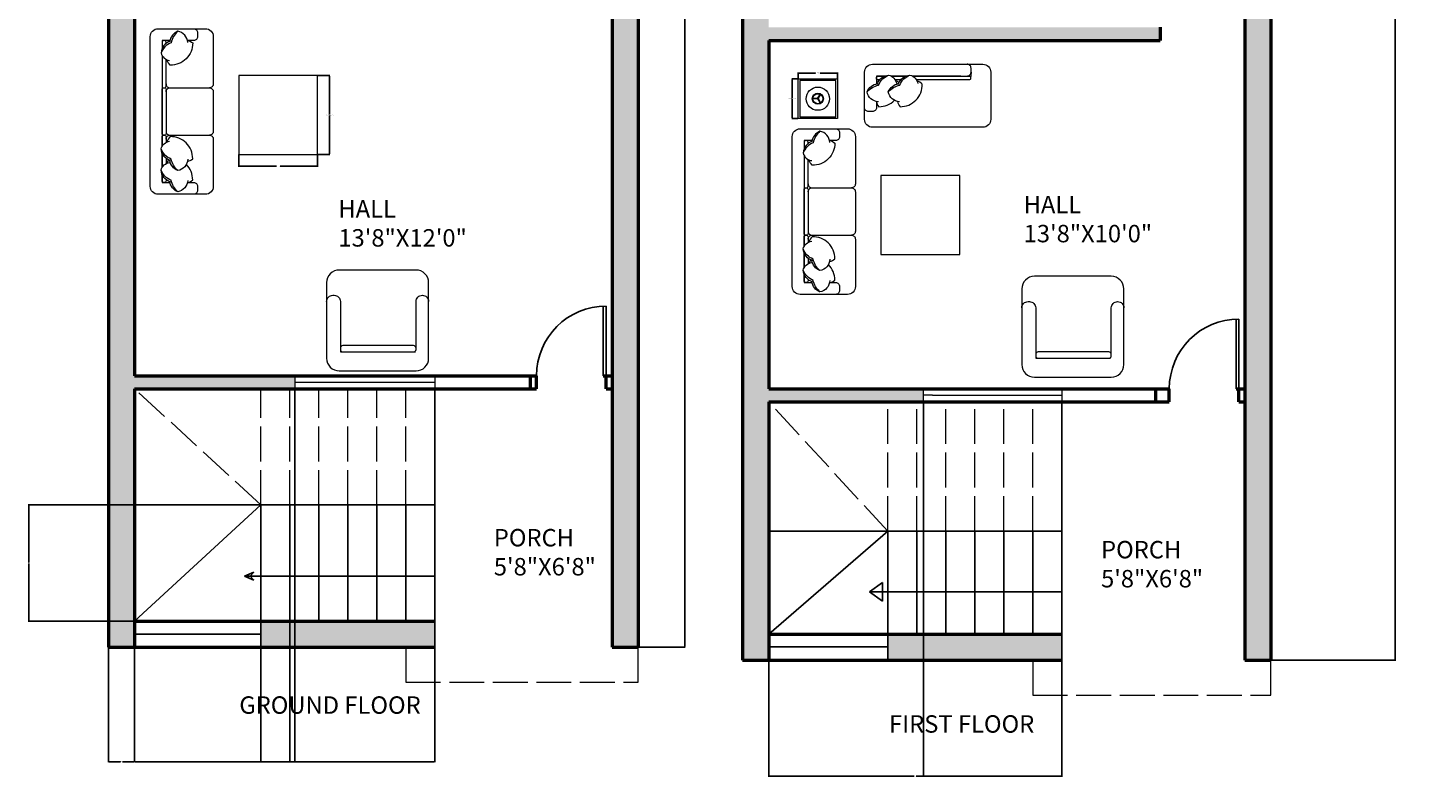
# Model space of a CAD drawing. Units: inches. Extents: x 3 to 485, y -522 to 42.
# Tile 1 of 6: x 3 to 485, y -522 to -264. Entities that reach past the tile are written whole.
import ezdxf

# ---------------------------------------------------------------- set-up
doc = ezdxf.new("R2010")
doc.units = ezdxf.units.IN
doc.header["$MEASUREMENT"] = 0
doc.linetypes.add('ACAD_ISO02W100', pattern=[15, 12, -3])
for name, color, linetype, lineweight in [('A-ANNO-DIMS', 2, 'Continuous', 18), ('A-ANNO-TEXT', 7, 'Continuous', 25), ('A-AREA-IDEN', 7, 'Continuous', 18), ('A-DOOR', 3, 'Continuous', 25), ('A-FLOR-OVHD', 7, 'ACAD_ISO02W100', 18), ('A-FLOR-STRS', 7, 'Continuous', 25), ('A-FLOR-STRS-OVHD', 7, 'ACAD_ISO02W100', 18), ('A-FURN', 8, 'Continuous', 18), ('A-GLAZ', 4, 'Continuous', 18), ('A-WALL', 7, 'Continuous', 50)]:
    doc.layers.add(name, color=color, linetype=linetype, lineweight=lineweight)
doc.layers.add('A-WALL-PATT', color=18, linetype='Continuous', lineweight=13, true_color=0x000000)
doc.styles.get("Standard").update_dxf_attribs({"font": 'arial.ttf'})
doc.dimstyles.get("Standard").update_dxf_attribs({"dimtxt": 0.18, "dimasz": 0.18, "dimexe": 0.18, "dimexo": 0.0625, "dimgap": 0.09, "dimtad": 0, "dimtih": 1, "dimtoh": 1, "dimdec": 0, "dimzin": 0, "dimdsep": 46, "dimlunit": 3, "dimtxsty": 'Standard', "dimcen": 0.09, "dimadec": 0, "dimazin": 0, "dimtfac": 1, "dimtdec": 0, "dimtofl": 0, "dimtmove": 0, "dimatfit": 3, "dimfxl": 1, "dimtolj": 1, "dimtzin": 0, "dimarcsym": 0})

# ---------------------------------------------------------------- blocks, each defined once
blk = doc.blocks.new('*D5')
at = {"layer": 'A-ANNO-DIMS', "color": 0, "lineweight": -2, "transparency": 16777216}
for p, q in [((212.85, 14), (229.02, 14)), ((228.84, 13.82), (228.84, -228.64)), ((228.84, -477.32), (228.84, -234.85)), ((212.85, -477.5), (229.02, -477.5))]:
    blk.add_line(p, q, dxfattribs=at)
at = {"layer": 'A-ANNO-DIMS', "color": 0, "transparency": 16777216}
for points in [[(228.81, 13.82), (228.87, 13.82), (228.84, 14)], [(228.81, -477.32), (228.87, -477.32), (228.84, -477.5)]]:
    blk.add_solid(points, dxfattribs=at)
at = {"layer": 'Defpoints', "color": 0, "transparency": 16777216}
for p in [(212.79, 14), (212.79, -477.5), (228.84, -477.5)]:
    blk.add_point(p, dxfattribs=at)
at = {"layer": 'A-ANNO-DIMS', "color": 0, "transparency": 16777216, "insert": (228.84, -231.75), "char_height": 6, "attachment_point": 5}
blk.add_mtext("\\A1;41'", dxfattribs=at)
blk = doc.blocks.new('DAY BED1')
at = {"color": 0}
blk.add_line((0.3, 0.25), (0.225, 0.255), dxfattribs=at)
blk.add_lwpolyline([(-0.3, 0, -0.414214), (-0.4, 0.1), (-0.4, 0.1, 0.317837), (-0.4, 0.1, -0.414214), (-0.4, 0.1), (-0.4, 0.1, 1.186185), (-0.4, 0.1, -0.414214), (-0.4, 0.1), (-0.4, 1.5, -0.414214), (-0.3, 1.6), (0.3, 1.6, -0.414214), (0.4, 1.5), (0.4, 0.1, -0.414214), (0.3, 0)], format="xyb", close=True, dxfattribs=at)
for points in [[(-0.073, 1.45), (-0.15, 1.45, -0.414214), (-0.2, 1.5), (-0.2, 1.55, -0.414214), (-0.15, 1.6)], [(-0.073, 1.45, 0.165541), (-0.139, 1.419, 0.200231), (-0.058, 1.221, 0.121523)], [(-0.076, 1.425, -0.356772), (0.05, 1.568, -0.249542), (0.154, 1.438, 9.61688)], [(0.05, 1.568, -0.14773), (0.136, 1.422, -0.213343), (0.262, 1.293, -0.178662)], [(0.143, 1.442, -0.306663), (0.262, 1.293, -0.30633), (0.154, 1.196, 0.872847)], [(0.25, 1.345), (0.25, 1.45), (0.152, 1.45, -0.414214)], [(0.2, 1.412), (0.2, 1.43, -0.414214), (0.22, 1.45), (0.23, 1.45, -0.414214), (0.25, 1.43)], [(0.25, 1.43), (0.25, 1.345, -0.414214)], [(-0.076, 1.156, -0.356772), (0.05, 1.299, -0.249542), (0.154, 1.169, 9.61688)], [(0.05, 1.299, -0.14773), (0.136, 1.153, -0.213343), (0.262, 1.024, -0.178662)], [(0.25, 1.262), (0.25, 1.075, -0.414214)], [(-0.073, 1.181, 0.165541), (-0.139, 1.15, 0.425989), (0.148, 0.869, 0.121523), (0.187, 0.936, -7.115464)], [(0.143, 1.173, -0.306663), (0.262, 1.024, -0.30633), (0.154, 0.926, 0.872847)], [(0.168, 1.163, 0.071865), (0.187, 1.205, -7.115464)], [(0.2, 1.142), (0.2, 1.211, -0.414214)], [(0.25, 0.992), (0.25, 0.275, -0.414214), (0.23, 0.255), (0.22, 0.255, -0.414214), (0.2, 0.275), (0.2, 0.942, -0.414214)], [(0.25, 0.377), (0.25, 0.3, 0.414214), (0.3, 0.25), (0.35, 0.25, 0.414214), (0.4, 0.3)]]:
    blk.add_lwpolyline(points, format="xyb", dxfattribs=at)
for points in [[(0.25, 1.075), (0.25, 1.262)], [(0.25, 0.377), (0.25, 0.992)]]:
    blk.add_lwpolyline(points, dxfattribs=at)
blk = doc.blocks.new('*D7')
at = {"layer": 'A-ANNO-DIMS', "color": 0, "lineweight": -2, "transparency": 16777216}
for p, q in [((430.85, 14), (473.81, 14)), ((473.63, 13.82), (473.63, -230.89)), ((473.63, -481.82), (473.63, -237.1)), ((430.85, -482), (473.81, -482))]:
    blk.add_line(p, q, dxfattribs=at)
at = {"layer": 'A-ANNO-DIMS', "color": 0, "transparency": 16777216}
for points in [[(473.6, 13.82), (473.66, 13.82), (473.63, 14)], [(473.6, -481.82), (473.66, -481.82), (473.63, -482)]]:
    blk.add_solid(points, dxfattribs=at)
at = {"layer": 'Defpoints', "color": 0, "transparency": 16777216}
for p in [(430.79, 14), (430.79, -482), (473.63, -482)]:
    blk.add_point(p, dxfattribs=at)
at = {"layer": 'A-ANNO-DIMS', "color": 0, "transparency": 16777216, "insert": (473.63, -234), "char_height": 6, "attachment_point": 5}
blk.add_mtext('\\A1;41\'-4"', dxfattribs=at)
blk = doc.blocks.new('LIVING-SIDE-TABLE')
for p, q in [((6.79, 6.87), (4.87, 6.87)), ((6.79, 6.7), (4.87, 6.7)), ((6.72, 6.83), (7.67, 8.49)), ((6.72, 6.75), (7.67, 5.09)), ((6.86, 6.75), (7.82, 8.41)), ((6.86, 6.83), (7.82, 5.17))]:
    blk.add_line(p, q)
at = {"ltscale": 0.03}
blk.add_lwpolyline([(13.58, 13.58), (13.58, 0), (0, 0), (0, 13.58)], close=True, dxfattribs=at)
blk.add_lwpolyline([(13.04, 0.54), (13.04, 13.04), (0.54, 13.04), (0.54, 0.54)], close=True)
for radius in [4, 1.92, 1.72]:
    blk.add_circle((6.79, 6.79), radius)
blk = doc.blocks.new('COFFEE-TABLE-SQUARE')
at = {"ltscale": 0.03}
blk.add_lwpolyline([(27.16, 0), (27.16, 27.16), (0, 27.16), (0, 0)], close=True, dxfattribs=at)
blk = doc.blocks.new('DOOR-SWING-24IN')
for p, q in [((-1, 0), (-1, 24)), ((0, 0), (0, 24))]:
    blk.add_line(p, q)
blk.add_arc((0, 0), 24, 90, 180)
blk = doc.blocks.new('*D26')
at = {"layer": 'A-ANNO-DIMS', "color": 0, "lineweight": -2, "transparency": 16777216}
for p, q in [((267.86, -281.8), (265.7, -281.8)), ((265.88, -281.98), (265.88, -288.41)), ((265.88, -295.2), (265.88, -288.77)), ((267.86, -295.38), (265.7, -295.38))]:
    blk.add_line(p, q, dxfattribs=at)
at = {"layer": 'A-ANNO-DIMS', "color": 0, "transparency": 16777216}
for points in [[(265.85, -281.98), (265.91, -281.98), (265.88, -281.8)], [(265.85, -295.2), (265.91, -295.2), (265.88, -295.38)]]:
    blk.add_solid(points, dxfattribs=at)
at = {"layer": 'Defpoints', "color": 0, "transparency": 16777216}
for p in [(265.88, -281.8), (267.92, -281.8), (267.92, -295.38)]:
    blk.add_point(p, dxfattribs=at)
at = {"layer": 'A-ANNO-DIMS', "color": 0, "transparency": 16777216, "insert": (265.88, -288.59), "char_height": 0.18, "attachment_point": 5}
blk.add_mtext('\\A1;SIDE TABLE 1\'-1 1/2" TYP.', dxfattribs=at)
blk = doc.blocks.new('*D27')
at = {"layer": 'A-ANNO-DIMS', "color": 0, "lineweight": -2, "transparency": 16777216}
for p, q in [((267.92, -281.74), (267.92, -279.58)), ((268.1, -279.76), (273.87, -279.76)), ((281.32, -279.76), (275.55, -279.76)), ((281.5, -281.74), (281.5, -279.58))]:
    blk.add_line(p, q, dxfattribs=at)
at = {"layer": 'A-ANNO-DIMS', "color": 0, "transparency": 16777216}
for points in [[(268.1, -279.73), (268.1, -279.79), (267.92, -279.76)], [(281.32, -279.73), (281.32, -279.79), (281.5, -279.76)]]:
    blk.add_solid(points, dxfattribs=at)
at = {"layer": 'Defpoints', "color": 0, "transparency": 16777216}
for p in [(281.5, -279.76), (267.92, -281.8), (281.5, -281.8)]:
    blk.add_point(p, dxfattribs=at)
at = {"layer": 'A-ANNO-DIMS', "color": 0, "transparency": 16777216, "insert": (274.71, -279.76), "char_height": 0.18, "attachment_point": 5}
blk.add_mtext('\\A1;1\'-1 1/2" TYP.', dxfattribs=at)
blk = doc.blocks.new('*D28')
at = {"layer": 'A-ANNO-DIMS', "color": 0, "lineweight": -2, "transparency": 16777216}
for p, q in [((102.43, -280.61), (106.62, -280.61)), ((106.44, -280.79), (106.44, -294)), ((106.44, -307.58), (106.44, -294.37)), ((102.43, -307.76), (106.62, -307.76))]:
    blk.add_line(p, q, dxfattribs=at)
at = {"layer": 'A-ANNO-DIMS', "color": 0, "transparency": 16777216}
for points in [[(106.41, -280.79), (106.47, -280.79), (106.44, -280.61)], [(106.41, -307.58), (106.47, -307.58), (106.44, -307.76)]]:
    blk.add_solid(points, dxfattribs=at)
at = {"layer": 'Defpoints', "color": 0, "transparency": 16777216}
for p in [(102.36, -280.61), (106.44, -280.61), (102.36, -307.76)]:
    blk.add_point(p, dxfattribs=at)
at = {"layer": 'A-ANNO-DIMS', "color": 0, "transparency": 16777216, "insert": (106.44, -294.18), "char_height": 0.18, "attachment_point": 5}
blk.add_mtext('\\A1;COFFEE TABLE 2\'-3" TYP.', dxfattribs=at)
blk = doc.blocks.new('*D29')
at = {"layer": 'A-ANNO-DIMS', "color": 0, "lineweight": -2, "transparency": 16777216}
for p, q in [((75.2, -307.83), (75.2, -312.02)), ((102.36, -307.83), (102.36, -312.02)), ((75.38, -311.84), (88.14, -311.84)), ((102.18, -311.84), (89.42, -311.84))]:
    blk.add_line(p, q, dxfattribs=at)
at = {"layer": 'A-ANNO-DIMS', "color": 0, "transparency": 16777216}
for points in [[(75.38, -311.81), (75.38, -311.87), (75.2, -311.84)], [(102.18, -311.81), (102.18, -311.87), (102.36, -311.84)]]:
    blk.add_solid(points, dxfattribs=at)
at = {"layer": 'Defpoints', "color": 0, "transparency": 16777216}
for p in [(75.2, -307.76), (102.36, -307.76), (102.36, -311.84)]:
    blk.add_point(p, dxfattribs=at)
at = {"layer": 'A-ANNO-DIMS', "color": 0, "transparency": 16777216, "insert": (88.78, -311.84), "char_height": 0.18, "attachment_point": 5}
blk.add_mtext('\\A1;2\'-3" TYP.', dxfattribs=at)
blk = doc.blocks.new('*D32')
at = {"layer": 'A-ANNO-DIMS', "color": 0, "lineweight": -2, "transparency": 16777216}
for p, q in [((30.29, -477.56), (30.29, -517.13)), ((39.29, -477.56), (39.29, -517.13)), ((30.47, -516.95), (34.46, -516.95)), ((39.11, -516.95), (35.12, -516.95))]:
    blk.add_line(p, q, dxfattribs=at)
at = {"layer": 'A-ANNO-DIMS', "color": 0, "transparency": 16777216}
for points in [[(30.47, -516.92), (30.47, -516.98), (30.29, -516.95)], [(39.11, -516.92), (39.11, -516.98), (39.29, -516.95)]]:
    blk.add_solid(points, dxfattribs=at)
at = {"layer": 'Defpoints', "color": 0, "transparency": 16777216}
for p in [(30.29, -477.5), (39.29, -477.5), (39.29, -516.95)]:
    blk.add_point(p, dxfattribs=at)
at = {"layer": 'A-ANNO-DIMS', "color": 0, "transparency": 16777216, "insert": (34.79, -516.95), "char_height": 0.18, "attachment_point": 5}
blk.add_mtext('\\A1;0\'-9"', dxfattribs=at)
blk = doc.blocks.new('*D33')
at = {"layer": 'A-ANNO-DIMS', "color": 0, "lineweight": -2, "transparency": 16777216}
for p, q in [((39.29, -468.56), (39.29, -517.13)), ((142.75, -468.56), (142.75, -517.13)), ((39.47, -516.95), (90.48, -516.95)), ((142.57, -516.95), (91.56, -516.95))]:
    blk.add_line(p, q, dxfattribs=at)
at = {"layer": 'A-ANNO-DIMS', "color": 0, "transparency": 16777216}
for points in [[(39.47, -516.92), (39.47, -516.98), (39.29, -516.95)], [(142.57, -516.92), (142.57, -516.98), (142.75, -516.95)]]:
    blk.add_solid(points, dxfattribs=at)
at = {"layer": 'Defpoints', "color": 0, "transparency": 16777216}
for p in [(39.29, -468.5), (142.75, -468.5), (142.75, -516.95)]:
    blk.add_point(p, dxfattribs=at)
at = {"layer": 'A-ANNO-DIMS', "color": 0, "transparency": 16777216, "insert": (91.02, -516.95), "char_height": 0.18, "attachment_point": 5}
blk.add_mtext('\\A1;8\'-7 1/2"', dxfattribs=at)
blk = doc.blocks.new('*D34')
at = {"layer": 'A-ANNO-DIMS', "color": 0, "lineweight": -2, "transparency": 16777216}
for p, q in [((257.79, -473.06), (257.79, -522.13)), ((358.77, -473.06), (358.77, -522.13)), ((257.97, -521.95), (307.95, -521.95)), ((358.59, -521.95), (308.61, -521.95))]:
    blk.add_line(p, q, dxfattribs=at)
at = {"layer": 'A-ANNO-DIMS', "color": 0, "transparency": 16777216}
for points in [[(257.97, -521.92), (257.97, -521.98), (257.79, -521.95)], [(358.59, -521.92), (358.59, -521.98), (358.77, -521.95)]]:
    blk.add_solid(points, dxfattribs=at)
at = {"layer": 'Defpoints', "color": 0, "transparency": 16777216}
for p in [(257.79, -473), (358.77, -473), (358.77, -521.95)]:
    blk.add_point(p, dxfattribs=at)
at = {"layer": 'A-ANNO-DIMS', "color": 0, "transparency": 16777216, "insert": (308.28, -521.95), "char_height": 0.18, "attachment_point": 5}
blk.add_mtext('\\A1;8\'-5"', dxfattribs=at)
blk = doc.blocks.new('*D35')
at = {"layer": 'A-ANNO-DIMS', "color": 0, "lineweight": -2, "transparency": 16777216}
for p, q in [((92.75, -468.56), (92.75, -517.13)), ((82.75, -473.06), (82.75, -517.13)), ((82.93, -516.95), (87.35, -516.95)), ((92.57, -516.95), (88.15, -516.95))]:
    blk.add_line(p, q, dxfattribs=at)
at = {"layer": 'A-ANNO-DIMS', "color": 0, "transparency": 16777216}
for points in [[(82.93, -516.92), (82.93, -516.98), (82.75, -516.95)], [(92.57, -516.92), (92.57, -516.98), (92.75, -516.95)]]:
    blk.add_solid(points, dxfattribs=at)
at = {"layer": 'Defpoints', "color": 0, "transparency": 16777216}
for p in [(92.75, -468.5), (82.75, -473), (92.75, -516.95)]:
    blk.add_point(p, dxfattribs=at)
at = {"layer": 'A-ANNO-DIMS', "color": 0, "transparency": 16777216, "insert": (87.75, -516.95), "char_height": 0.18, "attachment_point": 5}
blk.add_mtext('\\A1;0\'-10"', dxfattribs=at)
blk = doc.blocks.new('*D37')
at = {"layer": 'A-ANNO-DIMS', "color": 0, "lineweight": -2, "transparency": 16777216}
for p, q in [((94.55, -388.56), (94.55, -517.13)), ((142.75, -388.56), (142.75, -517.13)), ((94.73, -516.95), (118.32, -516.95)), ((142.57, -516.95), (118.99, -516.95))]:
    blk.add_line(p, q, dxfattribs=at)
at = {"layer": 'A-ANNO-DIMS', "color": 0, "transparency": 16777216}
for points in [[(94.73, -516.92), (94.73, -516.98), (94.55, -516.95)], [(142.57, -516.92), (142.57, -516.98), (142.75, -516.95)]]:
    blk.add_solid(points, dxfattribs=at)
at = {"layer": 'Defpoints', "color": 0, "transparency": 16777216}
for p in [(94.55, -388.5), (142.75, -388.5), (142.75, -516.95)]:
    blk.add_point(p, dxfattribs=at)
at = {"layer": 'A-ANNO-DIMS', "color": 0, "transparency": 16777216, "insert": (118.65, -516.95), "char_height": 0.18, "attachment_point": 5}
blk.add_mtext('\\A1;4\'-0"', dxfattribs=at)
blk = doc.blocks.new('*D38')
at = {"layer": 'A-ANNO-DIMS', "color": 0, "lineweight": -2, "transparency": 16777216}
for p, q in [((39.23, -428.5), (2.66, -428.5)), ((2.84, -428.68), (2.84, -448.31)), ((2.84, -468.32), (2.84, -448.68)), ((39.23, -468.5), (2.66, -468.5))]:
    blk.add_line(p, q, dxfattribs=at)
at = {"layer": 'A-ANNO-DIMS', "color": 0, "transparency": 16777216}
for points in [[(2.81, -428.68), (2.87, -428.68), (2.84, -428.5)], [(2.81, -468.32), (2.87, -468.32), (2.84, -468.5)]]:
    blk.add_solid(points, dxfattribs=at)
at = {"layer": 'Defpoints', "color": 0, "transparency": 16777216}
for p in [(2.84, -428.5), (39.29, -428.5), (39.29, -468.5)]:
    blk.add_point(p, dxfattribs=at)
at = {"layer": 'A-ANNO-DIMS', "color": 0, "transparency": 16777216, "insert": (2.84, -448.5), "char_height": 0.18, "attachment_point": 5}
blk.add_mtext('\\A1;3\'-4"', dxfattribs=at)
blk = doc.blocks.new('*D39')
at = {"layer": 'A-ANNO-DIMS', "color": 0, "lineweight": -2, "transparency": 16777216}
for p, q in [((311.15, -393.06), (311.15, -522.13)), ((358.77, -393.06), (358.77, -522.13)), ((311.33, -521.95), (334.35, -521.95)), ((358.59, -521.95), (335.57, -521.95))]:
    blk.add_line(p, q, dxfattribs=at)
at = {"layer": 'A-ANNO-DIMS', "color": 0, "transparency": 16777216}
for points in [[(311.33, -521.92), (311.33, -521.98), (311.15, -521.95)], [(358.59, -521.92), (358.59, -521.98), (358.77, -521.95)]]:
    blk.add_solid(points, dxfattribs=at)
at = {"layer": 'Defpoints', "color": 0, "transparency": 16777216}
for p in [(311.15, -393), (358.77, -393), (358.77, -521.95)]:
    blk.add_point(p, dxfattribs=at)
at = {"layer": 'A-ANNO-DIMS', "color": 0, "transparency": 16777216, "insert": (334.96, -521.95), "char_height": 0.18, "attachment_point": 5}
blk.add_mtext('\\A1;3\'-11 1/2"', dxfattribs=at)

msp = doc.modelspace()

# ---------------------------------------------------------------- hatches: boundary and pattern name
at = {"layer": 'A-WALL-PATT'}
h = msp.add_hatch(color=256, dxfattribs=at)
h.dxf.hatch_style = 1
h.paths.add_polyline_path([(177.79, -240), (177.79, -235.5), (39.29, -235.5), (39.29, 5), (87.29, 5), (87.29, -53), (91.79, -53), (91.79, 5), (203.79, 5), (203.79, -477.5), (212.79, -477.5), (212.79, 14), (30.29, 14), (30.29, -477.5), (39.29, -477.5), (39.29, -388.5), (94.55, -388.5), (94.55, -384), (39.29, -384), (39.29, -240)])
h.paths.add_polyline_path([(142.75, -477.5), (142.75, -468.5), (82.75, -468.5), (82.75, -477.5)], flags=17)
h.paths.add_polyline_path([(63.29, -79), (63.29, -83.5), (87.29, -83.5), (89.54, -83.5), (91.79, -83.5), (91.79, -77), (87.29, -77), (87.29, -79)], flags=17)
h.paths.add_polyline_path([(177.79, -139.5), (177.79, -135), (91.79, -135), (87.29, -135), (87.29, -139.5), (91.79, -139.5)], flags=17)
h = msp.add_hatch(color=256, dxfattribs=at)
h.dxf.hatch_style = 1
h.paths.add_polyline_path([(257.79, 5), (421.79, 5), (421.79, -482), (430.79, -482), (430.79, 14), (248.79, 14), (248.79, -482), (257.79, -482), (257.79, -393), (311.15, -393), (311.15, -388.5), (257.79, -388.5), (257.79, -268.5), (392.64, -268.5), (392.64, -264), (257.79, -264)])
h.paths.add_polyline_path([(358.77, -482), (358.77, -473), (298.77, -473), (298.77, -482)], flags=17)
h.paths.add_polyline_path([(298.14, -167.5), (298.14, -143.5), (293.64, -143.5), (293.64, -167.5), (293.64, -172), (392.64, -172), (392.64, -167.5), (392.64, -119.5), (388.14, -119.5), (388.14, -167.5)], flags=17)
h.paths.add_polyline_path([(362.14, -119.5), (362.14, -115), (293.64, -115), (293.64, -119.5)], flags=17)

# ---------------------------------------------------------------- linework, layer by layer
at = {"layer": 'A-FLOR-OVHD'}
for p, q in [((132.75, -477.5), (132.75, -489.5)), ((212.79, -489.5), (212.79, -477.5)), ((348.77, -482), (348.77, -494)), ((430.79, -494), (430.79, -482)), ((132.75, -489.5), (212.79, -489.5)), ((348.77, -494), (430.79, -494))]:
    msp.add_line(p, q, dxfattribs=at)
at = {"layer": 'A-FLOR-STRS'}
for p, q in [((142.75, -428.5), (39.29, -428.5)), ((82.75, -428.5), (39.29, -468.5)), ((82.75, -428.5), (82.75, -477.5)), ((92.75, -428.5), (92.75, -468.5)), ((102.75, -428.5), (102.75, -468.5)), ((112.75, -428.5), (112.75, -468.5)), ((122.75, -428.5), (122.75, -468.5)), ((132.75, -428.5), (132.75, -468.5)), ((142.75, -428.5), (142.75, -477.5)), ((358.77, -437.5), (257.79, -437.5)), ((298.77, -437.5), (257.79, -473)), ((298.77, -437.5), (298.77, -482)), ((308.77, -437.5), (308.77, -473)), ((318.77, -437.5), (318.77, -473)), ((328.77, -437.5), (328.77, -473)), ((328.77, -437.5), (328.77, -473)), ((338.77, -437.5), (338.77, -473)), ((348.77, -437.5), (348.77, -473)), ((358.77, -437.5), (358.77, -482)), ((77.2, -453), (80.33, -451.61)), ((142.75, -453), (77.2, -453)), ((77.2, -453), (80.33, -454.38)), ((80.33, -451.61), (79.17, -453)), ((80.33, -454.38), (79.17, -453)), ((292.51, -458.41), (296.98, -455.21)), ((296.98, -455.21), (296.98, -458.41)), ((358.77, -458.41), (292.51, -458.41)), ((292.51, -458.41), (296.98, -461.61)), ((296.98, -461.61), (296.98, -458.41)), ((82.75, -473), (39.29, -473)), ((298.77, -477.42), (257.79, -477.42))]:
    msp.add_line(p, q, dxfattribs=at)
at = {"layer": 'A-FLOR-STRS-OVHD'}
for p, q in [((82.75, -428.5), (39.29, -388.5)), ((82.75, -428.5), (82.75, -388.5)), ((92.75, -428.5), (92.75, -388.5)), ((102.75, -428.5), (102.75, -388.5)), ((112.75, -428.5), (112.75, -388.5)), ((122.75, -428.5), (122.75, -388.5)), ((132.75, -428.5), (132.75, -388.5)), ((142.75, -428.5), (142.75, -388.5)), ((298.77, -437.5), (257.79, -393)), ((298.77, -437.5), (298.77, -393)), ((308.77, -437.5), (308.77, -393)), ((318.77, -437.5), (318.77, -393)), ((328.77, -437.5), (328.77, -393)), ((338.77, -437.5), (338.77, -393)), ((348.77, -437.5), (348.77, -393)), ((358.77, -437.5), (358.77, -393))]:
    msp.add_line(p, q, dxfattribs=at)
at = {"layer": 'A-FURN', "ltscale": 0.03}
for points in [[(63.7, -264.48, -0.414214), (66.42, -267.2), (66.42, -283.49, -0.414214), (65.06, -284.85, -0.414214), (66.42, -286.21), (66.42, -299.79, -0.414214), (65.06, -301.15, -0.414214), (66.42, -302.51), (66.42, -318.8, -0.414214), (63.7, -321.52), (47.4, -321.52, -0.414214), (44.69, -318.8), (44.69, -267.2, -0.414214), (47.4, -264.48)], [(284.93, -298.95, -0.414214), (287.65, -301.66), (287.65, -317.96, -0.414214), (286.29, -319.32, -0.414214), (287.65, -320.67), (287.65, -334.25, -0.414214), (286.29, -335.61, -0.414214), (287.65, -336.97), (287.65, -353.26, -0.414214), (284.93, -355.98), (268.63, -355.98, -0.414214), (265.92, -353.26), (265.92, -301.66, -0.414214), (268.63, -298.95)], [(136.27, -382.33), (136.27, -382.33, 0.414214), (140.61, -377.99), (140.61, -351.93, 0.414214), (136.27, -347.59), (136.27, -347.59), (109.79, -347.59, 0.414214), (105.44, -351.93), (105.44, -377.99, 0.414214), (109.79, -382.33)], [(375.82, -384.51), (375.82, -384.51, 0.414214), (380.16, -380.17), (380.16, -354.12, 0.414214), (375.82, -349.77), (375.82, -349.77), (349.33, -349.77, 0.414214), (344.99, -354.12), (344.99, -380.17, 0.414214), (349.33, -384.51)]]:
    msp.add_lwpolyline(points, format="xyb", close=True, dxfattribs=at)
at = {"layer": 'A-FURN'}
for points in [[(59.63, -264.48, -0.414214), (60.98, -265.84), (60.98, -267.2, -0.414214), (59.63, -268.56), (57.52, -268.56)], [(54.18, -265.35, 0.14773), (51.85, -269.32, 0.213343), (48.42, -272.82, 0.178662)], [(51.66, -268.77, 0.306663), (48.42, -272.82, 0.30633), (51.38, -275.46, -0.872847)], [(50.12, -269.59), (50.12, -269.1, 0.414214), (49.58, -268.56), (49.31, -268.56, 0.414214), (48.76, -269.1)], [(48.76, -269.1), (48.76, -271.41, 0.414214)], [(57.52, -268.55, -0.165541), (59.32, -269.39, -0.425989), (51.54, -277.02, -0.121523), (50.46, -275.21, 7.115464)], [(57.6, -269.24, 0.356772), (54.18, -265.35, 0.249542), (51.36, -268.87, -9.61688)], [(48.76, -273.67), (48.76, -284.31, 0.414214), (49.31, -284.85), (49.58, -284.85, 0.414214), (50.12, -284.31), (50.12, -275.04, 0.414214)], [(50.12, -283.49, 0.414214), (51.48, -284.85), (65.06, -284.85, 0.414214)], [(50.12, -286.21, -0.414214), (51.48, -284.85)], [(280.86, -298.95, -0.414214), (282.21, -300.3), (282.21, -301.66, -0.414214), (280.86, -303.02), (278.75, -303.02)], [(51.66, -309.92, -0.306663), (48.42, -305.87, -0.30633), (51.38, -303.22, 0.872847)], [(48.76, -305.01), (48.76, -301.69, -0.414214), (49.31, -301.15), (49.58, -301.15, -0.414214), (50.12, -301.69), (50.12, -303.64, -0.414214)], [(50.12, -299.79, 0.414214), (51.48, -301.15)], [(50.12, -302.51, -0.414214), (51.48, -301.15), (65.06, -301.15, -0.414214)], [(57.52, -310.13, 0.165541), (59.32, -309.29, 0.425989), (51.54, -301.66, 0.121523), (50.46, -303.47, -7.115464)], [(275.41, -299.81, 0.14773), (273.08, -303.78, 0.213343), (269.65, -307.28, 0.178662)], [(272.89, -303.23, 0.306663), (269.65, -307.28, 0.30633), (272.61, -309.93, -0.872847)], [(271.35, -304.06), (271.35, -303.56, 0.414214), (270.81, -303.02), (270.54, -303.02, 0.414214), (269.99, -303.56)], [(269.99, -303.56), (269.99, -305.88, 0.414214)], [(278.75, -303.02, -0.165541), (280.55, -303.86, -0.425989), (272.77, -311.48, -0.121523), (271.69, -309.67, 7.115464)], [(278.83, -303.7, 0.356772), (275.41, -299.81, 0.249542), (272.59, -303.34, -9.61688)], [(54.18, -313.34, -0.14773), (51.85, -309.37, -0.213343), (48.42, -305.87, -0.178662)], [(48.76, -312.33), (48.76, -307.27, -0.414214)], [(269.99, -308.14), (269.99, -318.77, 0.414214), (270.54, -319.32), (270.81, -319.32, 0.414214), (271.35, -318.77), (271.35, -309.5, 0.414214)], [(51.66, -317.23, -0.306663), (48.42, -313.18, -0.30633), (51.38, -310.54, 0.872847)], [(54.18, -320.65, -0.14773), (51.85, -316.68, -0.213343), (48.42, -313.18, -0.178662)], [(50.12, -309.09), (50.12, -310.96, -0.414214)], [(51, -309.65, 0.071865), (50.46, -310.79, -7.115464)], [(57.6, -309.45, -0.356772), (54.18, -313.34, -0.249542), (51.36, -309.81, 9.61688)], [(57.52, -317.45, 0.165541), (59.32, -316.61, 0.200231), (57.13, -311.21, 0.121523)], [(48.76, -314.59), (48.76, -317.44), (51.43, -317.44, -0.414214)], [(48.76, -316.9), (48.76, -314.59, -0.414214)], [(50.12, -316.41), (50.12, -316.9, -0.414214), (49.58, -317.44), (49.31, -317.44, -0.414214), (48.76, -316.9)], [(57.6, -316.76, -0.356772), (54.18, -320.65, -0.249542), (51.36, -317.13, 9.61688)], [(57.52, -317.44), (59.63, -317.44, -0.414214), (60.98, -318.8), (60.98, -320.16, -0.414214), (59.63, -321.52)], [(271.35, -317.96, 0.414214), (272.71, -319.32), (286.29, -319.32, 0.414214)], [(271.35, -320.67, -0.414214), (272.71, -319.32)], [(269.99, -339.48), (269.99, -336.15, -0.414214), (270.54, -335.61), (270.81, -335.61, -0.414214), (271.35, -336.15), (271.35, -338.11, -0.414214)], [(271.35, -334.25, 0.414214), (272.71, -335.61)], [(271.35, -336.97, -0.414214), (272.71, -335.61), (286.29, -335.61, -0.414214)], [(278.75, -344.59, 0.165541), (280.55, -343.75, 0.425989), (272.77, -336.13, 0.121523), (271.69, -337.94, -7.115464)], [(272.89, -344.38, -0.306663), (269.65, -340.33, -0.30633), (272.61, -337.68, 0.872847)], [(275.41, -347.8, -0.14773), (273.08, -343.83, -0.213343), (269.65, -340.33, -0.178662)], [(269.99, -346.79), (269.99, -341.73, -0.414214)], [(272.89, -351.7, -0.306663), (269.65, -347.65, -0.30633), (272.61, -345, 0.872847)], [(271.35, -343.55), (271.35, -345.42, -0.414214)], [(272.23, -344.11, 0.071865), (271.69, -345.25, -7.115464)], [(278.83, -343.91, -0.356772), (275.41, -347.8, -0.249542), (272.59, -344.28, 9.61688)], [(278.75, -351.91, 0.165541), (280.55, -351.07, 0.200231), (278.36, -345.68, 0.121523)], [(275.41, -355.12, -0.14773), (273.08, -351.15, -0.213343), (269.65, -347.65, -0.178662)], [(269.99, -349.05), (269.99, -351.91), (272.66, -351.91, -0.414214)], [(269.99, -351.36), (269.99, -349.05, -0.414214)], [(271.35, -350.87), (271.35, -351.36, -0.414214), (270.81, -351.91), (270.54, -351.91, -0.414214), (269.99, -351.36)], [(278.83, -351.22, -0.356772), (275.41, -355.12, -0.249542), (272.59, -351.59, 9.61688)], [(278.75, -351.91), (280.86, -351.91, -0.414214), (282.21, -353.26), (282.21, -354.62, -0.414214), (280.86, -355.98)], [(105.44, -358.45, -0.414214), (107.61, -356.28), (108.05, -356.28, -0.414214), (110.22, -358.45), (110.22, -361.81)], [(136.27, -374.51), (136.27, -358.45, -0.414214), (138.44, -356.28), (138.44, -356.28, -0.414214), (140.61, -358.45)], [(344.99, -360.63, -0.414214), (347.16, -358.46), (347.59, -358.46, -0.414214), (349.77, -360.63), (349.77, -363.99)], [(375.82, -376.69), (375.82, -360.63, -0.414214), (377.99, -358.46), (377.99, -358.46, -0.414214), (380.16, -360.63)], [(120.58, -373.64), (111.09, -373.64, 0.414214), (110.22, -374.51), (110.22, -374.95, 0.414214), (111.09, -375.82)], [(111.09, -375.82), (118.4, -375.82, 0.414214)], [(118.4, -375.82), (135.4, -375.82, 0.414214), (136.27, -374.95), (136.27, -374.51, 0.414214), (135.4, -373.64), (120.58, -373.64, 0.414214)], [(360.13, -375.83), (350.63, -375.83, 0.414214), (349.77, -376.69), (349.77, -377.13, 0.414214), (350.63, -378)], [(357.94, -378), (374.95, -378, 0.414214), (375.82, -377.13), (375.82, -376.69, 0.414214), (374.95, -375.83), (360.13, -375.83, 0.414214)], [(350.63, -378), (357.94, -378, 0.414214)]]:
    msp.add_lwpolyline(points, format="xyb", dxfattribs=at)
for points in [[(51.43, -268.56), (48.76, -268.56), (48.76, -271.41)], [(48.76, -273.67), (48.76, -305.01)], [(272.66, -303.02), (269.99, -303.02), (269.99, -305.88)], [(48.76, -307.27), (48.76, -312.33)], [(269.99, -308.14), (269.99, -339.48)], [(269.99, -341.73), (269.99, -346.79)], [(110.22, -361.81), (110.22, -375.82), (118.4, -375.82)], [(349.77, -363.99), (349.77, -378), (357.94, -378)], [(118.4, -375.82), (136.05, -375.82)], [(357.94, -378), (375.6, -378)]]:
    msp.add_lwpolyline(points, dxfattribs=at)
for points in [[(48.76, -300.6), (48.76, -285.4, -0.414214), (49.31, -284.85), (49.58, -284.85, -0.414214), (50.12, -285.4), (50.12, -300.6, -0.414214), (49.58, -301.15), (49.31, -301.15, -0.414214)], [(269.99, -335.07), (269.99, -319.86, -0.414214), (270.54, -319.32), (270.81, -319.32, -0.414214), (271.35, -319.86), (271.35, -335.07, -0.414214), (270.81, -335.61), (270.54, -335.61, -0.414214)]]:
    msp.add_lwpolyline(points, format="xyb", close=True, dxfattribs=at)
at = {"layer": 'A-GLAZ'}
for p, q in [((94.55, -384), (94.55, -388.5)), ((142.75, -384), (142.75, -388.5)), ((94.55, -386.25), (142.75, -386.25)), ((311.15, -393), (311.15, -388.5)), ((358.77, -388.5), (358.77, -393)), ((314.18, -390.75), (311.15, -390.75)), ((314.18, -390.75), (358.77, -390.75))]:
    msp.add_line(p, q, dxfattribs=at)
at = {"layer": 'A-WALL'}
for p, q in [((30.29, 14), (30.29, -477.5)), ((212.79, 14), (212.79, -477.5)), ((248.79, 14), (248.79, -482)), ((430.79, 14), (430.79, -482)), ((203.79, 5), (203.79, -477.5)), ((421.79, 5), (421.79, -482)), ((39.29, -240), (39.29, -384)), ((392.64, -264), (392.64, -268.5)), ((257.79, -268.5), (392.64, -268.5)), ((257.79, -268.5), (257.79, -388.5)), ((39.29, -384), (177.79, -384)), ((175.63, -384), (175.63, -387.1)), ((177.79, -388.5), (177.79, -384)), ((200.79, -384), (203.79, -384)), ((201.79, -388.5), (201.79, -384)), ((39.29, -388.5), (177.79, -388.5)), ((39.29, -388.5), (39.29, -477.5)), ((175.63, -387.1), (175.63, -388.5)), ((201.79, -388.5), (203.79, -388.5)), ((257.79, -388.5), (395.79, -388.5)), ((391.04, -388.5), (391.04, -393)), ((395.79, -393), (395.79, -388.5)), ((418.79, -388.5), (421.79, -388.5)), ((419.79, -393), (419.79, -388.5)), ((257.79, -393), (395.79, -393)), ((257.79, -393), (257.79, -482)), ((419.79, -393), (421.79, -393)), ((39.29, -468.5), (142.75, -468.5)), ((30.29, -477.5), (142.75, -477.5)), ((203.79, -477.5), (212.79, -477.5)), ((257.79, -473), (358.77, -473)), ((248.79, -482), (358.77, -482)), ((421.79, -482), (430.79, -482))]:
    msp.add_line(p, q, dxfattribs=at)

# ---------------------------------------------------------------- block references
at = {"layer": 'A-DOOR'}
for p in [(201.79, -384), (419.79, -388.5)]:
    msp.add_blockref('DOOR-SWING-24IN', p, dxfattribs=at)
at = {"layer": 'A-FURN', "ltscale": 0.03, "xscale": 27.15874568996764, "yscale": 27.15874568996764, "zscale": 27.15874568996764, "rotation": 90}
msp.add_blockref('DAY BED1', (334.27, -287.57), dxfattribs=at)
at = {"layer": 'A-FURN'}
for name, p in [('COFFEE-TABLE-SQUARE', (75.2, -307.76)), ('LIVING-SIDE-TABLE', (267.92, -295.38)), ('COFFEE-TABLE-SQUARE', (296.44, -342.23))]:
    msp.add_blockref(name, p, dxfattribs=at)

# ---------------------------------------------------------------- texts
at = {"layer": 'A-ANNO-TEXT', "char_height": 6, "attachment_point": 1}
for s, insert in [('GROUND FLOOR', (75.38, -494.44)), ('FIRST FLOOR', (299.25, -500.95))]:
    msp.add_mtext(s, dxfattribs=dict(at, insert=insert))
at = {"layer": 'A-AREA-IDEN', "char_height": 6, "attachment_point": 1}
for s, insert in [('HALL\\P13\'8"X10\'0"', (345.62, -322.05)), ('HALL\\P13\'8"X12\'0"', (109.51, -323.52)), ('PORCH\\P5\'8"X6\'8"', (372.29, -440.91))]:
    msp.add_mtext(s, dxfattribs=dict(at, insert=insert))
at = {"layer": 'A-AREA-IDEN', "insert": (163.06, -436.79), "char_height": 6, "attachment_point": 1}
msp.add_mtext_dynamic_manual_height_columns('PORCH\\P5\'8"X6\'8"', width=0.8809, gutter_width=1, heights=[0], dxfattribs=at)

# ---------------------------------------------------------------- dimensions: what is measured, and where the dimension line sits
at = {"layer": 'A-ANNO-DIMS'}
for base, p1, p2, override, picture, middle in [((228.83525514, -477.49647159), (212.79082571, 14.00352841), (212.79082571, -477.49647159), {"dimtxt": 6, "dimclrd": 0, "dimclre": 0, "dimclrt": 0}, '*D5', (228.83525514, -231.74647159)), ((473.63, -482), (430.79, 14), (430.79, -482), {"dimtxt": 6, "dimclrd": 0, "dimclre": 0, "dimclrt": 0}, '*D7', (473.63, -234)), ((2.84, -428.5), (39.29, -468.5), (39.29, -428.5), {"dimdec": 1, "dimlfac": 1, "dimrnd": 0, "dimzin": 1, "dimdsep": 46, "dimlunit": 4, "dimfrac": 2}, '*D38', (2.84, -448.5))]:
    dim = msp.add_linear_dim(base=base, p1=p1, p2=p2, angle=90, dimstyle='Standard', override=override, dxfattribs=at)
    dim.commit()
    dim.dimension.update_dxf_attribs({"geometry": picture, "text_midpoint": middle})
for base, p1, p2, picture, middle in [((281.5, -279.76), (267.92, -281.8), (281.5, -281.8), '*D27', (274.71, -279.76)), ((102.36, -311.84), (75.2, -307.76), (102.36, -307.76), '*D29', (88.78, -311.84))]:
    dim = msp.add_linear_dim(base=base, p1=p1, p2=p2, text='<> TYP.', dimstyle='Standard', override={"dimdec": 1, "dimlfac": 1, "dimrnd": 0, "dimzin": 1, "dimdsep": 46, "dimlunit": 4, "dimfrac": 2}, dxfattribs=at)
    dim.commit()
    dim.dimension.update_dxf_attribs({"geometry": picture, "text_midpoint": middle})
for base, p1, p2, text, picture, middle in [((106.4374, -280.6054), (102.3636, -307.7641), (102.3636, -280.6054), 'COFFEE TABLE <> TYP.', '*D28', (106.4374, -294.1848)), ((265.88, -281.8), (267.92, -295.38), (267.92, -281.8), 'SIDE TABLE <> TYP.', '*D26', (265.88, -288.59))]:
    dim = msp.add_linear_dim(base=base, p1=p1, p2=p2, angle=90, text=text, dimstyle='Standard', override={"dimdec": 1, "dimlfac": 1, "dimrnd": 0, "dimzin": 1, "dimdsep": 46, "dimlunit": 4, "dimfrac": 2}, dxfattribs=at)
    dim.commit()
    dim.dimension.update_dxf_attribs({"geometry": picture, "text_midpoint": middle})
for base, p1, p2, picture, middle in [((142.75, -516.95), (94.55, -388.5), (142.75, -388.5), '*D37', (118.65, -516.95)), ((358.77, -521.95), (311.15, -393), (358.77, -393), '*D39', (334.96, -521.95)), ((142.75, -516.95), (39.29, -468.5), (142.75, -468.5), '*D33', (91.02, -516.95)), ((92.75, -516.95), (82.75, -473), (92.75, -468.5), '*D35', (87.75, -516.95)), ((39.29, -516.95), (30.29, -477.5), (39.29, -477.5), '*D32', (34.79, -516.95)), ((358.77, -521.95), (257.79, -473), (358.77, -473), '*D34', (308.28, -521.95))]:
    dim = msp.add_linear_dim(base=base, p1=p1, p2=p2, dimstyle='Standard', override={"dimdec": 1, "dimlfac": 1, "dimrnd": 0, "dimzin": 1, "dimdsep": 46, "dimlunit": 4, "dimfrac": 2}, dxfattribs=at)
    dim.commit()
    dim.dimension.update_dxf_attribs({"geometry": picture, "text_midpoint": middle})

doc.saveas('drawing.dxf')
